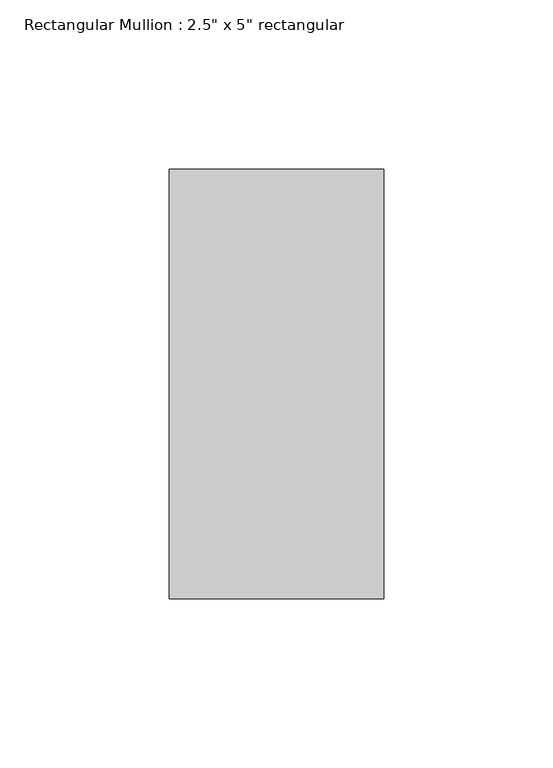
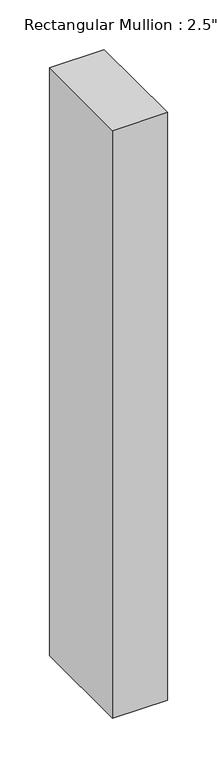
"""IFC4 building model written with IfcOpenShell, lengths in millimetres: member geometry."""

from ifc_helpers import new_model, si_unit, frame, origin, place, context, project, spatial, polyline, outline, extrude, source, transform, mapped, element, save


def member_47c7a801(model_context):
    return source(origin(), model_context, "Body", "SweptSolid", [
        extrude(outline(polyline([(0.0, 63.5), (0.0, -63.5), (-63.5, -63.5), (-63.5, 63.5), (0.0, 63.5)])), frame((0.0, 0.0, -721.1902035), z_axis=(0.0, 0.0, 1.0), x_axis=(1.0, 0.0, 0.0)), (0.0, 0.0, 1.0), 721.1902035),
    ])


if __name__ == "__main__":
    model = new_model("IFC4")
    model_context = context("Model", 3, world=origin())
    ifc_project = project(units=[si_unit("LENGTHUNIT", "METRE", prefix="MILLI")], contexts=[model_context])
    site = spatial("IfcSite", under=ifc_project)
    building = spatial("IfcBuilding", under=site)
    placement = place(None, origin())
    member_shape = member_47c7a801(model_context)
    element("IfcMember", 1, ObjectType="Rectangular Mullion : 2.5\" x 5\" rectangular", at=placement, inside=building, context=model_context, shape_type="MappedRepresentation", body=[
        mapped(member_shape, transform((0.0, 0.0, 0.0), x_axis=(1.0, 0.0, 0.0), y_axis=(0.0, 1.0, 0.0), z_axis=(0.0, 0.0, 1.0))),
    ])
    save(model, "model.ifc")

# Revit data of these elements
# Type "Rectangular Mullion : 2.5\" x 5\" rectangular"
#   built-in parameter 1007304 = 0.416667 (stored number, unit not read)
#   built-in parameter 1007301 = 0.104167 (stored number, unit not read)
#   built-in parameter 1007300 = 0.104167 (stored number, unit not read)
# Element 1 (IfcMember, "Rectangular Mullion : 2.5\" x 5\" rectangular")
#   Materials on its faces: "Aluminum"
# Materials
#   "Aluminum": class "Metal", colour RGB 247 247 247, transparency 0, Description = "Aluminum 6061", Cost = 0
